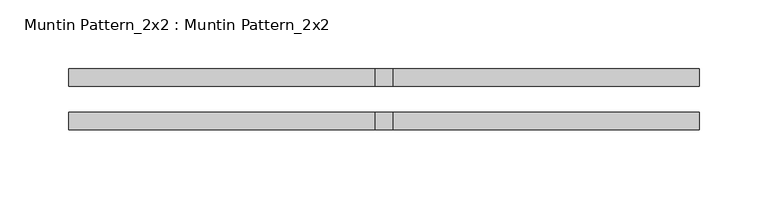
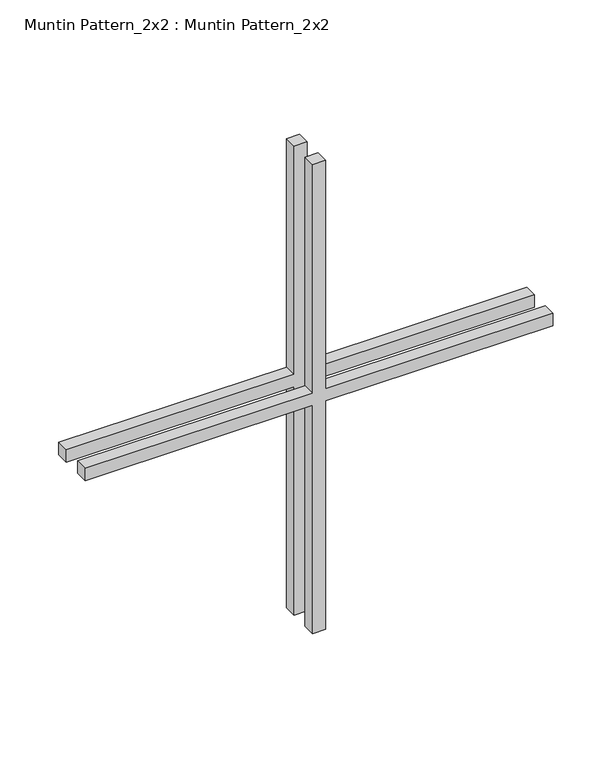
"""IFC4 building model written with IfcOpenShell, lengths in millimetres: proxy geometry, Muntin Pattern_2x2 : Muntin Pattern_2x2."""

from ifc_helpers import new_model, si_unit, frame, origin, place, context, project, spatial, polyline, outline, extrude, source, transform, mapped, element, save


def muntin_pattern_2x2_muntin_pattern_2x2_6213a163(model_context):
    return source(origin(), model_context, "Body", "SweptSolid", [
        extrude(outline(polyline([(249.2375, -6.35), (249.2375, -229.39375), (236.5375, -229.39375), (236.5375, -6.35), (0.0, -6.35), (0.0, 6.35), (236.5375, 6.35), (236.5375, 229.39375), (249.2375, 229.39375), (249.2375, 6.35), (485.775, 6.35), (485.775, -6.35), (249.2375, -6.35)])), frame((0.0, -22.225, 0.0), z_axis=(0.0, 1.0, 0.0), x_axis=(0.0, 0.0, 1.0)), (0.0, 0.0, 1.0), 12.7),
        extrude(outline(polyline([(249.2375, -6.35), (249.2375, -229.39375), (236.5375, -229.39375), (236.5375, -6.35), (0.0, -6.35), (0.0, 6.35), (236.5375, 6.35), (236.5375, 229.39375), (249.2375, 229.39375), (249.2375, 6.35), (485.775, 6.35), (485.775, -6.35), (249.2375, -6.35)])), frame((0.0, 9.525, 0.0), z_axis=(0.0, 1.0, 0.0), x_axis=(0.0, 0.0, 1.0)), (0.0, 0.0, 1.0), 12.7),
    ])


if __name__ == "__main__":
    model = new_model("IFC4")
    model_context = context("Model", 3, world=origin())
    ifc_project = project(units=[si_unit("LENGTHUNIT", "METRE", prefix="MILLI")], contexts=[model_context])
    site = spatial("IfcSite", under=ifc_project)
    building = spatial("IfcBuilding", under=site)
    placement = place(None, origin())
    muntin_pattern_2x2_muntin_pattern_2x2_shape = muntin_pattern_2x2_muntin_pattern_2x2_6213a163(model_context)
    element("IfcBuildingElementProxy", 1, Name="Muntin Pattern_2x2 : Muntin Pattern_2x2", ObjectType="Muntin Pattern_2x2 : Muntin Pattern_2x2", at=placement, inside=building, context=model_context, shape_type="MappedRepresentation", body=[
        mapped(muntin_pattern_2x2_muntin_pattern_2x2_shape, transform((0.0, 0.0, 0.0), x_axis=(1.0, 0.0, 0.0), y_axis=(0.0, 1.0, 0.0), z_axis=(0.0, 0.0, 1.0))),
    ])
    save(model, "model.ifc")

# Revit data of these elements
# Type "Muntin Pattern_2x2 : Muntin Pattern_2x2"
#   Width [instance default] = 4' - 0"
#   Thickness = 0' - 0 1/2"
#   Height [instance default] = 4' - 0"
#   Distance = 0' - 0 3/4"
#   Interior Material [instance default] = none
#   Exterior Material [instance default] = none
#   Default Elevation = 0
# Element 1 (IfcBuildingElementProxy, "Muntin Pattern_2x2 : Muntin Pattern_2x2")
#   Width = 1' - 6 1/16"
#   Height = 1' - 7 1/8"
#   Interior Material = Wood - Stained
#   Exterior Material = Clad - White
#   Materials on its faces: "Clad - White", "Wood - Stained"
# Materials
#   "Clad - White": class "Wood", colour RGB 242 242 238, transparency 0, Cost = 0
#   "Wood - Stained": class "Wood", colour RGB 224 178 126, transparency 0, Cost = 0
